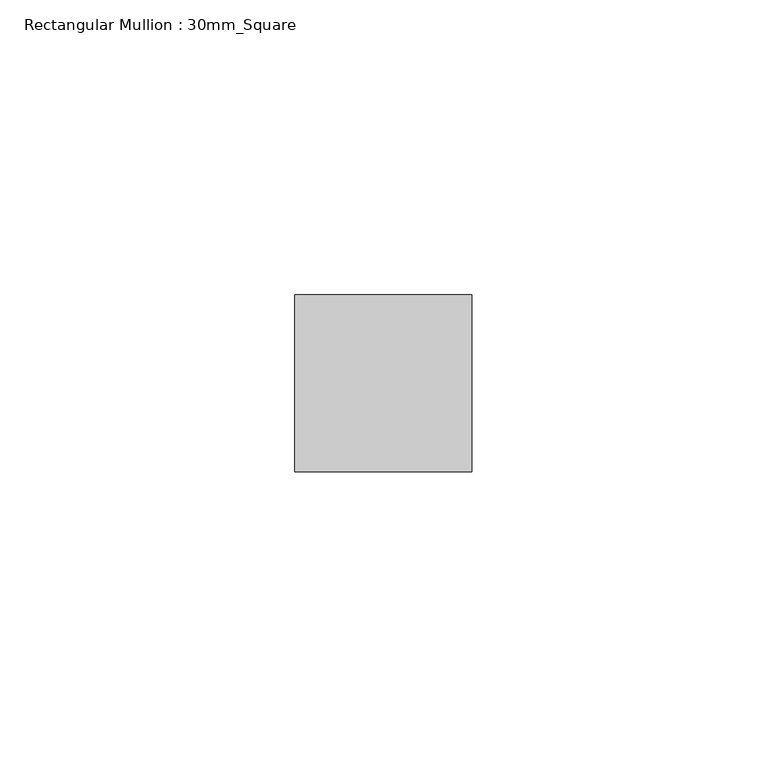
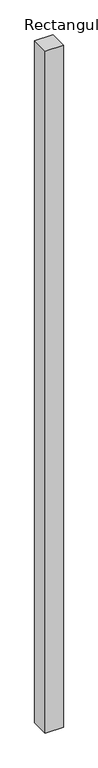
"""IFC4 building model written with IfcOpenShell, lengths in millimetres: member geometry, Rectangular Mullion : 30mm_Square."""

from ifc_helpers import new_model, si_unit, frame, origin, place, context, project, spatial, polyline, outline, extrude, source, transform, mapped, element, save


def rectangular_mullion_30mm_square_cc57b060(model_context):
    return source(origin(), model_context, "Body", "SweptSolid", [
        extrude(outline(polyline([(0.0, 15.0), (0.0, -15.0), (-30.0, -15.0), (-30.0, 15.0), (0.0, 15.0)])), frame((0.0, 0.0, -1191.1333334), z_axis=(0.0, 0.0, 1.0), x_axis=(1.0, 0.0, 0.0)), (0.0, 0.0, 1.0), 1191.1333334),
    ])


if __name__ == "__main__":
    model = new_model("IFC4")
    model_context = context("Model", 3, world=origin())
    ifc_project = project(units=[si_unit("LENGTHUNIT", "METRE", prefix="MILLI")], contexts=[model_context])
    site = spatial("IfcSite", under=ifc_project)
    building = spatial("IfcBuilding", under=site)
    placement = place(None, origin())
    rectangular_mullion_30mm_square_shape = rectangular_mullion_30mm_square_cc57b060(model_context)
    element("IfcMember", 1, ObjectType="Rectangular Mullion : 30mm_Square", at=placement, inside=building, context=model_context, shape_type="MappedRepresentation", body=[
        mapped(rectangular_mullion_30mm_square_shape, transform((0.0, 0.0, 0.0), x_axis=(1.0, 0.0, 0.0), y_axis=(0.0, 1.0, 0.0), z_axis=(0.0, 0.0, 1.0))),
    ])
    save(model, "model.ifc")

# Revit data of these elements
# Type "Rectangular Mullion : 30mm_Square"
#   Keynote = "H11"
#   built-in parameter 1007304 = 0.0984252 (stored number, unit not read)
#   built-in parameter 1007301 = 0.0492126 (stored number, unit not read)
#   built-in parameter 1007300 = 0.0492126 (stored number, unit not read)
# Element 1 (IfcMember, "Rectangular Mullion : 30mm_Square")
#   Materials on its faces: "Aluminium"
# Materials
#   "Aluminium": class "Metal", colour RGB 247 247 247, transparency 0, Description = "Aluminium 6061", Cost = 0
